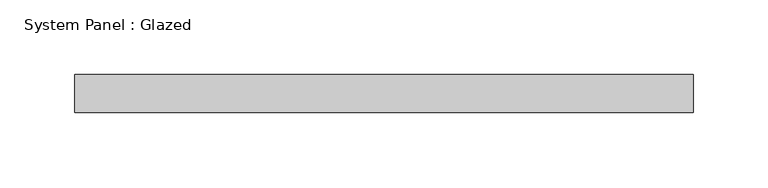
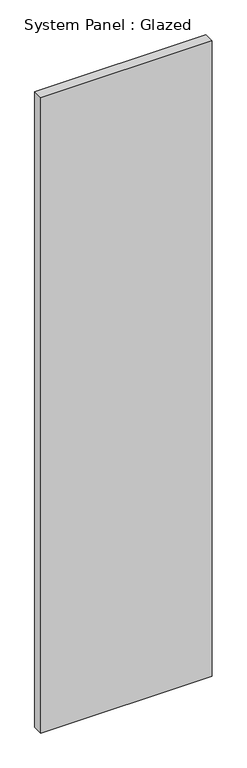
"""IFC4 building model written with IfcOpenShell, lengths in millimetres: plate geometry, System Panel : Glazed."""

from ifc_helpers import new_model, si_unit, origin, origin_with_axes, place, context, project, spatial, polyline, outline, extrude, source, transform, mapped, element, save


def system_panel_glazed_3b3b315d(model_context):
    return source(origin(), model_context, "Body", "SweptSolid", [
        extrude(outline(polyline([(206.375, 19.05), (-206.375, 19.05), (-206.375, 44.45), (206.375, 44.45), (206.375, 19.05)])), origin_with_axes(), (0.0, 0.0, 1.0), 1620.5125275),
    ])


if __name__ == "__main__":
    model = new_model("IFC4")
    model_context = context("Model", 3, world=origin())
    ifc_project = project(units=[si_unit("LENGTHUNIT", "METRE", prefix="MILLI")], contexts=[model_context])
    site = spatial("IfcSite", under=ifc_project)
    building = spatial("IfcBuilding", under=site)
    placement = place(None, origin())
    system_panel_glazed_shape = system_panel_glazed_3b3b315d(model_context)
    element("IfcPlate", 1, ObjectType="System Panel : Glazed", at=placement, inside=building, context=model_context, shape_type="MappedRepresentation", body=[
        mapped(system_panel_glazed_shape, transform((0.0, 0.0, 0.0), x_axis=(1.0, 0.0, 0.0), y_axis=(0.0, 1.0, 0.0), z_axis=(0.0, 0.0, 1.0))),
    ])
    save(model, "model.ifc")

# Revit data of these elements
# Type "System Panel : Glazed"
#   Construction Type Id = "GSP4R"
#   Analytic Construction = "1/8 in Pilkington single glazing"
#   Visual Light Transmittance = 0.9
#   Solar Heat Gain Coefficient = 0.86
#   Heat Transfer Coefficient (U) = 1.18115 BTU/(h·ft²·°F)
#   Define Thermal Properties by = 1
# Element 1 (IfcPlate, "System Panel : Glazed")
#   Materials on its faces: "Glass"
# Materials
#   "Glass": class "Glass", colour RGB 0 128 192, transparency 0.75, Description = "Soda Lime Glass", Cost = 0
